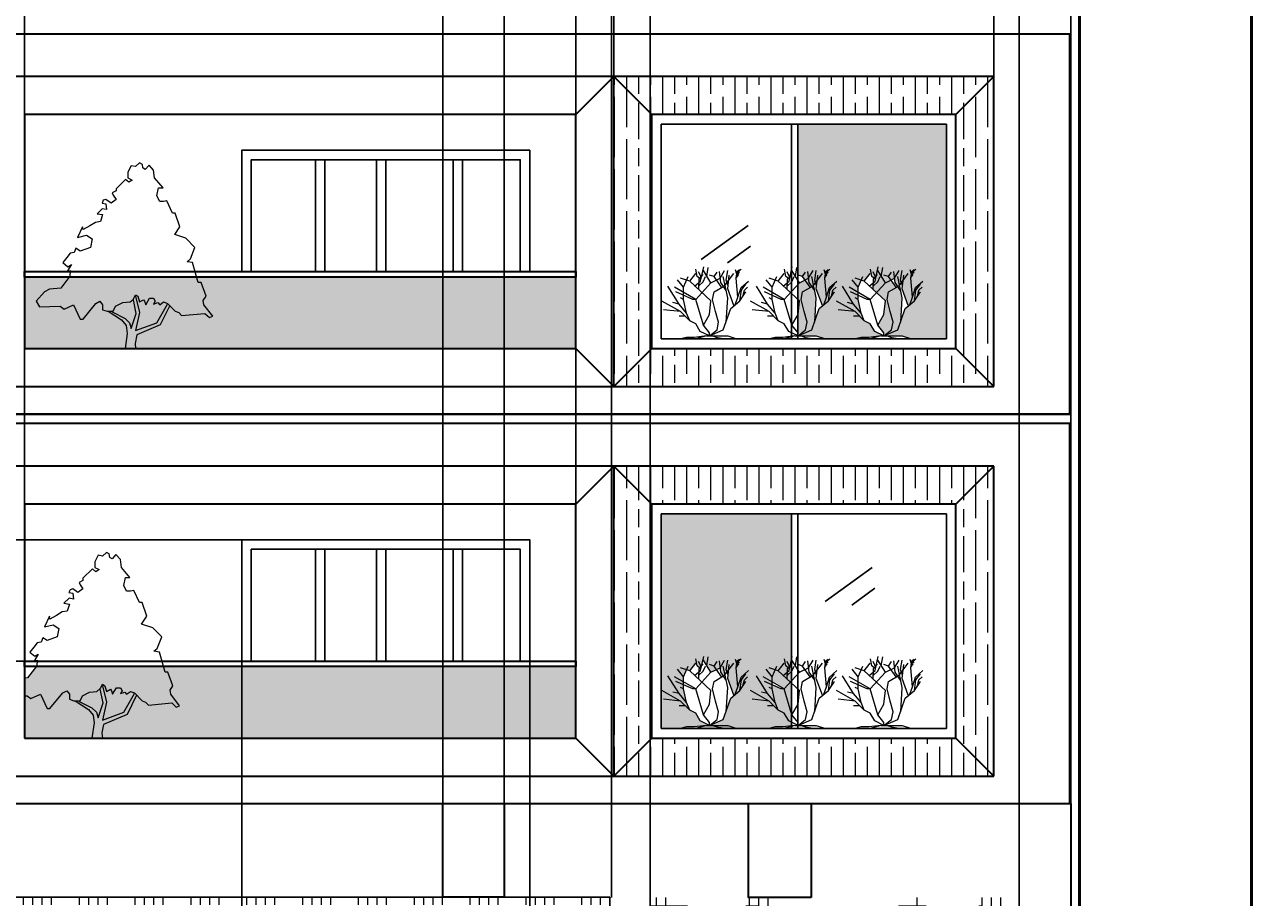
# Model space of a CAD drawing. Units: inches. Extents: x -97 to 1206, y -378 to 680.
# Tile 3 of 6: x 194 to 581, y -25 to 251. Entities that reach past the tile are written whole.
import ezdxf

# ---------------------------------------------------------------- set-up
doc = ezdxf.new("R2010")
doc.units = ezdxf.units.IN
doc.header["$MEASUREMENT"] = 0
for name, color, linetype, lineweight in [('A-ANNO-DIMS', 2, 'Continuous', 18), ('A-DOOR', 3, 'Continuous', 25), ('A-ELEV', 7, 'Continuous', 35), ('A-ELEV-PATT', 252, 'Continuous', 13), ('A-GLAZ', 4, 'Continuous', 25), ('A-WALL', 7, 'Continuous', 50), ('L-PLNT', 82, 'Continuous', 13)]:
    doc.layers.add(name, color=color, linetype=linetype, lineweight=lineweight)
doc.styles.get("Standard").update_dxf_attribs({"font": 'arial.ttf'})
doc.dimstyles.get("Standard").update_dxf_attribs({"dimtxt": 0.18, "dimasz": 0.18, "dimexe": 0.18, "dimexo": 0.0625, "dimgap": 0.09, "dimtad": 0, "dimtih": 1, "dimtoh": 1, "dimdec": 4, "dimzin": 0, "dimdsep": 46, "dimtxsty": 'Standard', "dimcen": 0.09, "dimadec": 0, "dimazin": 0, "dimtfac": 1, "dimtdec": 4, "dimtofl": 0, "dimtmove": 0, "dimatfit": 3, "dimfxl": 1, "dimtolj": 1, "dimtzin": 0, "dimarcsym": 0})
pattern_1 = [(45, (-208.809, -191.922), (8.48528, 0), [5, -7]), (45, (-206.6876, -191.922), (8.48528, 0), [2, -10]), (45, (-208.809, -189.8007), (8.48528, 0), [2, -10])]

# ---------------------------------------------------------------- blocks, each defined once
blk = doc.blocks.new('*U2')
for p, q in [((-16.8, 16.32), (-15.36, 19.68)), ((-14.88, 18.24), (-12.96, 20.64)), ((-12.471, 19.775), (-12.898, 22.044)), ((-11.677, 19.071), (-12.471, 19.775)), ((-11.28, 19.619), (-12.104, 21.184)), ((-11.921, 18.836), (-10.64, 20.401)), ((-11.433, 18.289), (-10.457, 22.749)), ((-10.579, 18.054), (-9.846, 19.697)), ((-8.16, 17.76), (-10.56, 21.6)), ((-9.48, 19.775), (-8.992, 22.592)), ((-7.2, 19.68), (-8.64, 20.16)), ((-7.2, 19.68), (-6.24, 21.12)), ((-4.8, 16.32), (-7.2, 19.68)), ((-5.086, 17.741), (-5.513, 21.34)), ((-5.28, 19.2), (-3.84, 21.6)), ((-2.88, 12.96), (-4.32, 19.68)), ((-3.84, 16.8), (-0.96, 20.64)), ((-3.377, 18.602), (-2.888, 21.575)), ((-2.88, 15.84), (-2.4, 20.16)), ((-0.508, 21.888), (-0.081, 20.558)), ((-0.203, 19.149), (0.102, 21.34)), ((-0.142, 19.384), (0.59, 20.401)), ((-0.02, 20.01), (0.896, 21.105)), ((0.041, 20.714), (1.384, 22.044)), ((0.102, 21.34), (0.835, 21.888)), ((-18.24, 11.04), (-21.755, 16.655)), ((-12.96, 12.48), (-19.68, 16.32)), ((-16.8, 16.32), (-18.72, 18.72)), ((-14.88, 18.24), (-17.76, 19.2)), ((-16.8, 12.48), (-16.8, 16.32)), ((-8.16, 12), (-14.88, 18.24)), ((-13.325, 16.724), (-11.433, 18.289)), ((-12.96, 12.48), (-8.16, 17.76)), ((-12.043, 15.628), (-11.921, 18.836)), ((-11.982, 16.802), (-10.579, 18.054)), ((-8.16, 17.76), (-5.28, 19.2)), ((-7.2, 14.88), (-3.84, 16.8)), ((-3.377, 15.315), (-5.086, 17.819)), ((-2.766, 16.802), (-3.377, 18.602)), ((-0.96, 10.56), (-2.88, 15.84)), ((0.346, 13.203), (-0.203, 19.149)), ((0.346, 13.203), (1.323, 16.254)), ((1.323, 16.254), (3.642, 18.289)), ((1.44, 15.36), (2.88, 17.28)), ((2.4, 15.36), (3.36, 16.32)), ((-17.76, 8.64), (-23.663, 11.961)), ((-13.92, 12.48), (-19.2, 14.88)), ((-16.8, 12.48), (-17.76, 12.96)), ((-15.84, 8.16), (-16.8, 12.48)), ((-12.96, 12.48), (-13.92, 12.48)), ((-10.56, 4.32), (-12.96, 12.48)), ((-8.64, 7.68), (-8.16, 12)), ((-7.68, 12.48), (-7.2, 14.88)), ((-6.72, 8.64), (-7.68, 12.48)), ((-3.36, 5.28), (-2.88, 12.96)), ((-1.92, 9.6), (0.96, 12)), ((-0.48, 10.8), (0.346, 13.203)), ((0.96, 12), (1.44, 15.36)), ((0.96, 12), (2.88, 14.88)), ((1.92, 13.44), (2.4, 15.36)), ((-17.76, 8.64), (-23.128, 9.222)), ((-18.24, 11.04), (-20.16, 11.52)), ((-15.84, 8.16), (-18.24, 11.04)), ((-14.88, 5.76), (-17.76, 8.64)), ((-14.88, 5.76), (-15.84, 8.16)), ((-5.76, 5.28), (-6.72, 8.64)), ((-4.32, 2.88), (-1.92, 9.6)), ((-16.32, 7.2), (-18.24, 7.2)), ((-12.96, 4.8), (-14.88, 5.76)), ((-11.52, 2.4), (-12.96, 4.8)), ((-10.56, 4.32), (-8.64, 7.68)), ((-8.64, 1.92), (-10.56, 4.32)), ((-6.24, 2.88), (-5.76, 5.28)), ((-15.84, 0.48), (-17.76, 0)), ((-13.44, 0.48), (-15.84, 0.48)), ((-9.6, 0.96), (-13.44, 0.48)), ((-9.6, 0.96), (-12.96, 0)), ((-8.64, 0.96), (-11.52, 2.4)), ((-9.6, 0.96), (-7.68, 0.96)), ((-8.64, 0.96), (-4.32, 2.88)), ((-8.64, 0.96), (-6.24, 2.88)), ((-8.64, 0.96), (-8.64, 1.92)), ((-8.64, 0.96), (-2.88, 0.96)), ((-7.68, 0.96), (-6.24, 0.48)), ((-6.24, 0.48), (-3.36, 0)), ((-2.88, 0.96), (0, 0))]:
    blk.add_line(p, q)
blk = doc.blocks.new('*U3')
for points in [[(22.0124, 137.721), (18.5475, 141.5624), (15.5282, 138.2446), (13.8028, 139.3505), (13.3714, 142.1153), (11.2148, 143.2214), (8.1954, 140.4564), (4.7447, 141.0094), (2.1567, 136.0326), (2.1567, 131.6088), (5.6074, 129.9499), (3.0193, 128.2909), (0.4313, 130.5029), (-6.9015, 123.3141), (-6.9015, 121.6552), (-9.9208, 119.9963), (-9.0581, 118.3373), (-6.9015, 115.0195), (-10.7835, 112.2546), (-14.6656, 115.0195), (-16.8222, 114.4665), (-17.6849, 112.2546), (-14.6656, 111.7016), (-14.2342, 107.2778), (-17.6065, 107.8307), (-21.5669, 103.9599), (-17.2536, 103.4069), (-18.9789, 97.8771), (-22.8609, 97.3241), (-27.1743, 94.5593), (-32.3504, 91.7944), (-32.7817, 94.0063), (-36.6638, 85.7116), (-29.7624, 87.3705), (-25.449, 84.6056), (-26.743, 77.9699), (-34.507, 75.205), (-37.9578, 77.4169), (-39.2518, 74.099), (-42.2711, 73.5461), (-44.8592, 70.2282), (-47.8786, 66.3574), (-43.9965, 63.0395), (-41.4085, 64.6985), (-44.3346, 59.8898), (-42.2089, 60.1377), (-42.5159, 55.7849), (-49.6039, 46.4502), (-58.2307, 45.8972), (-62.1127, 43.6853), (-68.5828, 36.4966), (-65.9947, 32.0727), (-50.0352, 32.6257), (-47.0159, 30.4138), (-39.6831, 33.7317), (-34.507, 22.6721), (-32.3504, 22.6721), (-22.4296, 34.8376), (-19.4102, 36.4966), (-17.2536, 33.7317), (-17.2536, 29.8608), (-13.8028, 28.7549), (-9.0581, 28.7549), (-7.3328, 32.6257), (-1.7254, 35.3906), (3.8821, 35.9436), (6.4701, 38.1555), (6.9014, 38.7085), (8.1954, 41.4734), (9.9208, 40.3674), (11.2148, 35.9436), (14.2341, 37.6025), (15.0968, 36.4966), (15.9595, 33.7317), (18.9789, 38.7085), (21.9982, 38.7085), (23.2922, 36.4966), (21.9982, 34.2847), (25.4489, 35.3906), (26.743, 33.7317), (29.7623, 35.9436), (32.7817, 34.8376), (38.8204, 28.7549), (41.4084, 27.6489), (43.5651, 25.437), (61.6813, 27.0959), (65.132, 23.7781), (67.7201, 24.884), (60.8186, 33.7317), (60.3873, 37.0495), (62.544, 40.3674), (58.662, 50.874), (56.5053, 50.874), (52.1919, 66.3574), (47.8785, 66.9103), (50.4665, 69.1222), (53.9172, 77.9699), (47.0158, 85.1586), (38.3891, 87.9235), (42.2711, 94.0063)], [(42.2711, 94.0063), (38.8204, 104.5129), (36.6637, 104.5129), (32.3503, 113.9135), (29.7623, 113.3605), (26.743, 113.3605), (24.5862, 117.7844), (25.8802, 123.8671), (29.331, 123.8671), (22.8609, 131.6088), (21.9982, 137.6916)], [(8.1954, 40.3674), (11.2148, 27.6489), (8.1954, 13.8245), (24.5862, 19.9072), (32.7817, 34.2847)], [(-12.9401, 28.7549), (-2.588, 22.1191), (0.8626, 17.6953), (1.7253, 11.6125), (0, 0)], [(-9.9208, 28.2019), (0, 23.2251), (3.4507, 19.9072), (4.7447, 15.4834), (8.6267, 27.0959), (6.4701, 37.6025)], [(34.5071, 33.1787), (27.1743, 18.2483), (9.0581, 10.5066), (7.7641, 3.8708), (8.1954, 0)]]:
    blk.add_lwpolyline(points)
blk = doc.blocks.new('FACADE-SURROUND')
for p, q in [((432, 97.83), (0, 97.83)), ((0, 97.83), (0, 0)), ((12, 85.83), (0, 97.83)), ((300, 85.83), (312, 97.83)), ((312, 0), (312, 97.83)), ((312, 0), (312, 97.83)), ((312, 97.83), (324, 85.83)), ((432, 97.83), (420, 85.83)), ((432, 0), (432, 97.83)), ((12, 85.83), (12, 12)), ((108, 85.83), (12, 85.83)), ((300, 85.83), (126, 85.83)), ((126, 85.83), (126, 12)), ((300, 12), (300, 85.83)), ((324, 12), (324, 85.83)), ((420, 85.83), (324, 85.83)), ((420, 12), (420, 85.83)), ((12, 12), (0, 0)), ((12, 12), (108, 12)), ((126, 12), (300, 12)), ((300, 12), (312, 0)), ((312, 0), (324, 12)), ((324, 12), (420, 12)), ((432, 0), (420, 12)), ((0, 0), (432, 0))]:
    blk.add_line(p, q)
blk = doc.blocks.new('WIN-1500')
for p, q in [((90, 67.83), (0, 67.83)), ((0, 67.83), (0, 0)), ((90, 67.83), (90, 0)), ((0, 0), (90, 0))]:
    blk.add_line(p, q)
blk = doc.blocks.new('*D21')
at = {"layer": 'A-ANNO-DIMS', "color": 0, "lineweight": -2, "transparency": 16777216}
for p, q in [((379.25, -24.78), (379.25, 679.54)), ((379.43, 679.36), (451.27, 679.36)), ((524.01, 679.36), (452.18, 679.36)), ((524.19, -24.78), (524.19, 679.54))]:
    blk.add_line(p, q, dxfattribs=at)
at = {"layer": 'A-ANNO-DIMS', "color": 0, "transparency": 16777216}
for points in [[(379.43, 679.39), (379.43, 679.33), (379.25, 679.36)], [(524.01, 679.39), (524.01, 679.33), (524.19, 679.36)]]:
    blk.add_solid(points, dxfattribs=at)
at = {"layer": 'Defpoints', "color": 0, "transparency": 16777216}
for p in [(524.19, 679.36), (379.25, -24.84), (524.19, -24.84)]:
    blk.add_point(p, dxfattribs=at)
at = {"layer": 'A-ANNO-DIMS', "color": 0, "transparency": 16777216, "insert": (451.72, 679.36), "char_height": 0.18, "attachment_point": 5}
blk.add_mtext('\\A1;144.94', dxfattribs=at)
blk = doc.blocks.new('*D38')
at = {"layer": 'A-ANNO-DIMS', "color": 0, "lineweight": -2, "transparency": 16777216}
for p, q in [((391.36, -84.5), (391.36, 679.54)), ((391.54, 679.36), (449.18, 679.36)), ((507.74, 679.36), (450.1, 679.36)), ((507.92, -84.5), (507.92, 679.54))]:
    blk.add_line(p, q, dxfattribs=at)
at = {"layer": 'A-ANNO-DIMS', "color": 0, "transparency": 16777216}
for points in [[(391.54, 679.39), (391.54, 679.33), (391.36, 679.36)], [(507.74, 679.39), (507.74, 679.33), (507.92, 679.36)]]:
    blk.add_solid(points, dxfattribs=at)
at = {"layer": 'Defpoints', "color": 0, "transparency": 16777216}
for p in [(507.92, 679.36), (391.36, -84.57), (507.92, -84.57)]:
    blk.add_point(p, dxfattribs=at)
at = {"layer": 'A-ANNO-DIMS', "color": 0, "transparency": 16777216, "insert": (449.64, 679.36), "char_height": 0.18, "attachment_point": 5}
blk.add_mtext('\\A1;116.56', dxfattribs=at)
blk = doc.blocks.new('*D40')
at = {"layer": 'A-ANNO-DIMS', "color": 0, "lineweight": -2, "transparency": 16777216}
for p, q in [((193.93, 99.46), (193.93, 679.54)), ((194.11, 679.36), (280.65, 679.36)), ((367.75, 679.36), (281.21, 679.36)), ((367.93, 99.46), (367.93, 679.54))]:
    blk.add_line(p, q, dxfattribs=at)
at = {"layer": 'A-ANNO-DIMS', "color": 0, "transparency": 16777216}
for points in [[(194.11, 679.39), (194.11, 679.33), (193.93, 679.36)], [(367.75, 679.39), (367.75, 679.33), (367.93, 679.36)]]:
    blk.add_solid(points, dxfattribs=at)
at = {"layer": 'Defpoints', "color": 0, "transparency": 16777216}
for p in [(367.93, 679.36), (193.93, 99.4), (367.93, 99.4)]:
    blk.add_point(p, dxfattribs=at)
at = {"layer": 'A-ANNO-DIMS', "color": 0, "transparency": 16777216, "insert": (280.93, 679.36), "char_height": 0.18, "attachment_point": 5}
blk.add_mtext('\\A1;174', dxfattribs=at)
blk = doc.blocks.new('*D43')
at = {"layer": 'A-ANNO-DIMS', "color": 0, "lineweight": -2, "transparency": 16777216}
for p, q in [((262.49, 49.82), (262.49, -377.59)), ((353.38, 49.82), (353.38, -377.59)), ((262.67, -377.41), (307.54, -377.41)), ((353.2, -377.41), (308.33, -377.41))]:
    blk.add_line(p, q, dxfattribs=at)
at = {"layer": 'A-ANNO-DIMS', "color": 0, "transparency": 16777216}
for points in [[(262.67, -377.38), (262.67, -377.44), (262.49, -377.41)], [(353.2, -377.38), (353.2, -377.44), (353.38, -377.41)]]:
    blk.add_solid(points, dxfattribs=at)
at = {"layer": 'Defpoints', "color": 0, "transparency": 16777216}
for p in [(262.49, 49.88), (353.38, 49.88), (353.38, -377.41)]:
    blk.add_point(p, dxfattribs=at)
at = {"layer": 'A-ANNO-DIMS', "color": 0, "transparency": 16777216, "insert": (307.94, -377.41), "char_height": 0.18, "attachment_point": 5}
blk.add_mtext('\\A1;90.88', dxfattribs=at)
blk = doc.blocks.new('*D44')
at = {"layer": 'A-ANNO-DIMS', "color": 0, "lineweight": -2, "transparency": 16777216}
for p, q in [((262.43, 88.15), (-96.59, 88.15)), ((-96.41, 87.97), (-96.41, 69.2)), ((-96.41, 50.06), (-96.41, 68.83)), ((262.43, 49.88), (-96.59, 49.88))]:
    blk.add_line(p, q, dxfattribs=at)
at = {"layer": 'A-ANNO-DIMS', "color": 0, "transparency": 16777216}
for points in [[(-96.44, 87.97), (-96.38, 87.97), (-96.41, 88.15)], [(-96.44, 50.06), (-96.38, 50.06), (-96.41, 49.88)]]:
    blk.add_solid(points, dxfattribs=at)
at = {"layer": 'Defpoints', "color": 0, "transparency": 16777216}
for p in [(-96.41, 88.15), (262.49, 88.15), (262.49, 49.88)]:
    blk.add_point(p, dxfattribs=at)
at = {"layer": 'A-ANNO-DIMS', "color": 0, "transparency": 16777216, "insert": (-96.41, 69.01), "char_height": 0.18, "attachment_point": 5}
blk.add_mtext('\\A1;38.266', dxfattribs=at)
blk = doc.blocks.new('*D47')
at = {"layer": 'A-ANNO-DIMS', "color": 0, "lineweight": -2, "transparency": 16777216}
for p, q in [((184.83, -24.66), (184.83, 679.54)), ((185.01, 679.36), (255.01, 679.36)), ((325.75, 679.36), (255.75, 679.36)), ((325.93, -24.66), (325.93, 679.54))]:
    blk.add_line(p, q, dxfattribs=at)
at = {"layer": 'A-ANNO-DIMS', "color": 0, "transparency": 16777216}
for points in [[(185.01, 679.39), (185.01, 679.33), (184.83, 679.36)], [(325.75, 679.39), (325.75, 679.33), (325.93, 679.36)]]:
    blk.add_solid(points, dxfattribs=at)
at = {"layer": 'Defpoints', "color": 0, "transparency": 16777216}
for p in [(325.93, 679.36), (184.83, -24.73), (325.93, -24.73)]:
    blk.add_point(p, dxfattribs=at)
at = {"layer": 'A-ANNO-DIMS', "color": 0, "transparency": 16777216, "insert": (255.38, 679.36), "char_height": 0.18, "attachment_point": 5}
blk.add_mtext('\\A1;141.1', dxfattribs=at)
blk = doc.blocks.new('*D48')
at = {"layer": 'A-ANNO-DIMS', "color": 0, "lineweight": -2, "transparency": 16777216}
for p, q in [((325.93, -24.66), (325.93, 679.54)), ((326.11, 679.36), (335.23, 679.36)), ((345.13, 679.36), (336, 679.36)), ((345.31, -24.66), (345.31, 679.54))]:
    blk.add_line(p, q, dxfattribs=at)
at = {"layer": 'A-ANNO-DIMS', "color": 0, "transparency": 16777216}
for points in [[(326.11, 679.39), (326.11, 679.33), (325.93, 679.36)], [(345.13, 679.39), (345.13, 679.33), (345.31, 679.36)]]:
    blk.add_solid(points, dxfattribs=at)
at = {"layer": 'Defpoints', "color": 0, "transparency": 16777216}
for p in [(345.31, 679.36), (325.93, -24.73), (345.31, -24.73)]:
    blk.add_point(p, dxfattribs=at)
at = {"layer": 'A-ANNO-DIMS', "color": 0, "transparency": 16777216, "insert": (335.62, 679.36), "char_height": 0.18, "attachment_point": 5}
blk.add_mtext('\\A1;19.38', dxfattribs=at)
blk = doc.blocks.new('*D58')
at = {"layer": 'A-ANNO-DIMS', "color": 0, "lineweight": -2, "transparency": 16777216}
for p, q in [((379.93, 234.46), (379.93, 679.54)), ((380.11, 679.36), (439.47, 679.36)), ((499.75, 679.36), (440.38, 679.36)), ((499.93, 234.46), (499.93, 679.54))]:
    blk.add_line(p, q, dxfattribs=at)
at = {"layer": 'A-ANNO-DIMS', "color": 0, "transparency": 16777216}
for points in [[(380.11, 679.39), (380.11, 679.33), (379.93, 679.36)], [(499.75, 679.39), (499.75, 679.33), (499.93, 679.36)]]:
    blk.add_solid(points, dxfattribs=at)
at = {"layer": 'Defpoints', "color": 0, "transparency": 16777216}
for p in [(499.93, 679.36), (379.93, 234.4), (499.93, 234.4)]:
    blk.add_point(p, dxfattribs=at)
at = {"layer": 'A-ANNO-DIMS', "color": 0, "transparency": 16777216, "insert": (439.93, 679.36), "char_height": 0.18, "attachment_point": 5}
blk.add_mtext('\\A1;120.00', dxfattribs=at)

msp = doc.modelspace()

# ---------------------------------------------------------------- hatches: boundary and pattern name
at = {"layer": 'A-ELEV-PATT'}
h = msp.add_hatch(dxfattribs=at)
h.set_pattern_fill('GOST_GLASS', color=256)
h.set_pattern_definition(pattern_1)
h.paths.add_polyline_path([(441.8335, 588.3966), (394.9261, 588.3966), (394.9261, 520.5671), (441.8335, 520.5671)])
h.paths.add_polyline_path([(484.9261, 465.3966), (443.8021, 465.3966), (443.8021, 397.5671), (484.9261, 397.5671)])
h.paths.add_polyline_path([(441.8335, 342.3966), (394.9261, 342.3966), (394.9261, 274.5671), (441.8335, 274.5671)])
h.paths.add_polyline_path([(484.9261, 219.3966), (438.0187, 219.3966), (438.0187, 171.7458), (439.5149, 171.2471), (440.2728, 170.186), (438.5549, 169.3271), (438.0187, 168.7372), (438.0187, 164.065), (438.5549, 163.5671), (438.0187, 158.741), (438.0187, 153.5574), (438.6415, 152.7789), (438.0749, 152.5271), (443.8349, 152.5271), (446.7149, 151.5671), (456.0952, 151.5671), (458.0152, 152.0471), (460.4152, 152.0471), (465.0232, 152.6231), (462.3352, 153.9671), (460.8952, 156.3671), (458.9752, 157.3271), (458.0152, 159.7271), (457.0552, 164.0471), (457.0552, 167.8871), (458.0152, 170.1271), (458.9752, 169.8071), (461.1593, 172.5372), (461.3842, 171.3421), (462.1483, 170.6646), (462.7637, 171.4165), (462.4222, 169.8561), (461.8969, 169.4216), (461.8114, 167.1735), (465.6952, 163.5671), (465.2152, 159.2471), (463.2952, 155.8871), (465.7818, 152.7789), (465.2152, 152.5271), (470.9752, 152.5271), (473.8552, 151.5671), (484.9261, 151.5671)])
h.paths.add_polyline_path([(473.7595, 171.4865), (473.9183, 171.6764), (473.8259, 171.964)], flags=16)
h.paths.add_polyline_path([(468.5752, 170.7671), (468.5927, 170.7962), (468.758, 169.4025), (469.6192, 168.1408), (470.0152, 168.3671), (471.2674, 170.0367), (470.9752, 167.4071), (472.9399, 162.0043), (471.9352, 161.1671), (470.517, 157.1962), (470.9752, 164.5271), (470.4671, 166.8984), (469.6192, 168.1408), (469.09, 167.8384), (467.4131, 170.186)], flags=16)
h.paths.add_polyline_path([(446.6192, 171.4865), (446.778, 171.6764), (446.6857, 171.964)], flags=16)
h.paths.add_polyline_path([(444.7949, 161.1671), (443.3768, 157.1962), (443.8349, 164.5271), (443.3268, 166.8984), (442.4789, 168.1408), (442.8749, 168.3671), (444.1271, 170.0367), (443.8349, 167.4071), (445.7996, 162.0043)], flags=16)
h.paths.add_polyline_path([(436.0501, 96.3966), (394.9261, 96.3966), (394.9261, 28.5671), (436.0501, 28.5671)])
h.paths.add_polyline_path([(418.6647, 48.4865), (418.8235, 48.6764), (418.7312, 48.964)], flags=16)
h.paths.add_polyline_path([(408.0905, 50.343), (410.6005, 46.3271), (413.4805, 47.7671), (413.4979, 47.7962), (413.6633, 46.4025), (414.5244, 45.1408), (414.9205, 45.3671), (416.1726, 47.0367), (415.8805, 44.4071), (417.8451, 39.0043), (416.8405, 38.1671), (414.4405, 31.4471), (410.1205, 29.5271), (407.2405, 30.9671), (405.8005, 33.3671), (403.8805, 34.3271), (402.9205, 36.7271), (401.9605, 41.0471), (401.9605, 44.8871), (402.9205, 47.1271), (403.8805, 46.8071), (406.0646, 49.5372), (406.2895, 48.3421), (407.0535, 47.6646), (407.6689, 48.4165)], flags=16)
h.paths.add_polyline_path([(406.7167, 44.1735), (410.6005, 40.5671), (410.1205, 36.2471), (408.2005, 32.8871), (405.8005, 41.0471), (407.761, 43.2037), (405.4765, 45.3251), (406.8021, 46.4216)], flags=0)
h.paths.add_polyline_path([(429.9149, 43.2414), (433.7549, 41.0471), (432.7949, 41.0471), (429.9149, 42.3562)], flags=16)
h = msp.add_hatch(dxfattribs=at)
h.set_pattern_fill('GOST_GLASS', color=256)
h.set_pattern_definition(pattern_1)
h.paths.add_polyline_path([(225.9926, 155.8067), (224.5809, 157.6166), (220.3456, 160.3315), (219.9926, 160.3315), (218.5808, 160.7839), (218.5808, 162.3676), (217.6985, 163.4988), (216.4631, 162.8201), (212.4043, 157.8428), (211.522, 157.8428), (209.4043, 162.3676), (206.4043, 161.0102), (205.169, 161.9151), (198.6395, 161.6889), (197.5807, 163.4988), (200.2278, 166.4399), (201.816, 167.3448), (205.3454, 167.5711), (208.0494, 171.1321), (193.9261, 171.1321), (193.9261, 148.5671), (225.6397, 148.5671), (226.3455, 153.3181)])
h.paths.add_polyline_path([(228.9926, 165.5349), (229.6985, 165.0825), (230.2279, 163.2726), (231.4632, 163.9513), (231.8162, 163.4988), (232.1691, 162.3676), (233.4044, 164.4038), (234.6397, 164.4038), (235.1691, 163.4988), (234.6397, 162.5939), (236.0515, 163.0463), (236.5809, 162.3676), (237.8162, 163.2726), (239.0515, 162.8201), (241.5221, 160.3315), (242.5809, 159.879), (243.4633, 158.974), (250.8751, 159.6527), (252.2869, 158.2953), (253.3457, 158.7478), (250.5222, 162.3676), (250.3457, 163.725), (251.2281, 165.0825), (249.6398, 169.381), (248.7575, 169.381), (248.2696, 171.1321), (208.0494, 171.1321), (205.3454, 167.5711), (201.816, 167.3448), (200.2278, 166.4399), (197.5807, 163.4988), (198.6395, 161.6889), (205.169, 161.9151), (206.4043, 161.0102), (209.4043, 162.3676), (211.522, 157.8428), (212.4043, 157.8428), (216.4631, 162.8201), (217.6985, 163.4988), (218.5808, 162.3676), (218.5808, 160.7839), (219.9926, 160.3315), (221.9338, 160.3315), (222.6396, 161.9151), (224.9338, 163.0463), (227.228, 163.2726), (228.2868, 164.1775), (228.4632, 164.4038)])
h.paths.add_polyline_path([(236.7574, 156.033), (239.7468, 162.1197), (239.0515, 162.8201), (237.8162, 163.2726), (236.5809, 162.3676), (236.0515, 163.0463), (234.6397, 162.5939), (235.1691, 163.4988), (234.6397, 164.4038), (233.4044, 164.4038), (232.1691, 162.3676), (231.8162, 163.4988), (231.4632, 163.9513), (230.2279, 163.2726), (229.6985, 165.0825), (228.9926, 165.5349), (228.4632, 164.4038), (228.2868, 164.1775), (227.228, 163.2726), (224.9338, 163.0463), (222.6396, 161.9151), (221.9338, 160.3315), (220.3456, 160.3315), (224.5809, 157.6166), (225.9926, 155.8067), (226.3455, 153.3181), (225.6397, 148.5671), (228.9926, 148.5671), (228.8162, 150.1507), (229.3456, 152.8656)])
h.paths.add_polyline_path([(367.9261, 171.1321), (248.2696, 171.1321), (248.7575, 169.381), (249.6398, 169.381), (251.2281, 165.0825), (250.3457, 163.725), (250.5222, 162.3676), (253.3457, 158.7478), (252.2869, 158.2953), (250.8751, 159.6527), (243.4633, 158.974), (242.5809, 159.879), (241.5221, 160.3315), (239.7468, 162.1197), (236.7574, 156.033), (229.3456, 152.8656), (228.8162, 150.1507), (228.9926, 148.5671), (367.9261, 148.5671)])
h.paths.add_polyline_path([(367.9261, 48.1321), (237.8147, 48.1321), (238.3026, 46.381), (239.1849, 46.381), (240.7732, 42.0825), (239.8908, 40.725), (240.0673, 39.3676), (242.8908, 35.7478), (241.832, 35.2953), (240.4202, 36.6527), (233.0084, 35.974), (232.126, 36.879), (231.0672, 37.3315), (229.2919, 39.1197), (226.3025, 33.033), (218.8907, 29.8656), (218.3613, 27.1507), (218.5377, 25.5671), (367.9261, 25.5671)])
h.paths.add_polyline_path([(226.3025, 33.033), (229.2919, 39.1197), (228.5966, 39.8201), (227.3613, 40.2726), (226.126, 39.3676), (225.5966, 40.0463), (224.1848, 39.5939), (224.7142, 40.4988), (224.1848, 41.4038), (222.9495, 41.4038), (221.7142, 39.3676), (221.3613, 40.4988), (221.0083, 40.9513), (219.7731, 40.2726), (219.2436, 42.0825), (218.5377, 42.5349), (218.0083, 41.4038), (217.8319, 41.1775), (216.7731, 40.2726), (214.4789, 40.0463), (212.1847, 38.9151), (211.4789, 37.3315), (209.8907, 37.3315), (214.126, 34.6166), (215.5377, 32.8067), (215.8907, 30.3181), (215.1848, 25.5671), (218.5377, 25.5671), (218.3613, 27.1507), (218.8907, 29.8656)])
h.paths.add_polyline_path([(239.1849, 46.381), (238.3026, 46.381), (237.8147, 48.1321), (197.5945, 48.1321), (194.8905, 44.5711), (193.9261, 44.5093), (193.9261, 38.8878), (194.7141, 38.9151), (195.9494, 38.0102), (198.9494, 39.3676), (201.0671, 34.8428), (201.9494, 34.8428), (206.0083, 39.8201), (207.2436, 40.4988), (208.1259, 39.3676), (208.1259, 37.7839), (209.5377, 37.3315), (211.4789, 37.3315), (212.1847, 38.9151), (214.4789, 40.0463), (216.7731, 40.2726), (217.8319, 41.1775), (218.0083, 41.4038), (218.5377, 42.5349), (219.2436, 42.0825), (219.7731, 40.2726), (221.0083, 40.9513), (221.3613, 40.4988), (221.7142, 39.3676), (222.9495, 41.4038), (224.1848, 41.4038), (224.7142, 40.4988), (224.1848, 39.5939), (225.5966, 40.0463), (226.126, 39.3676), (227.3613, 40.2726), (228.5966, 39.8201), (231.0672, 37.3315), (232.126, 36.879), (233.0084, 35.974), (240.4202, 36.6527), (241.832, 35.2953), (242.8908, 35.7478), (240.0673, 39.3676), (239.8908, 40.725), (240.7732, 42.0825)])
h.paths.add_polyline_path([(215.5377, 32.8067), (214.126, 34.6166), (209.8907, 37.3315), (209.5377, 37.3315), (208.1259, 37.7839), (208.1259, 39.3676), (207.2436, 40.4988), (206.0083, 39.8201), (201.9494, 34.8428), (201.0671, 34.8428), (198.9494, 39.3676), (195.9494, 38.0102), (194.7141, 38.9151), (193.9261, 38.8878), (193.9261, 25.5671), (215.1848, 25.5671), (215.8907, 30.3181)])
h.paths.add_polyline_path([(336.7518, 280.6166), (332.5165, 283.3315), (332.1636, 283.3315), (330.7518, 283.7839), (330.7518, 285.3676), (329.8694, 286.4988), (328.6341, 285.8201), (324.5753, 280.8428), (323.6929, 280.8428), (321.5753, 285.3676), (318.5752, 284.0102), (317.3399, 284.9151), (310.8105, 284.6889), (309.7516, 286.4988), (312.3987, 289.4399), (313.987, 290.3448), (317.5164, 290.5711), (320.2203, 294.1321), (199.9261, 294.1321), (199.9261, 271.5671), (337.8106, 271.5671), (338.5165, 276.3181), (338.1636, 278.8067)])
h.paths.add_polyline_path([(321.5753, 408.3676), (318.5752, 407.0102), (317.3399, 407.9151), (310.8105, 407.6889), (309.7516, 409.4988), (312.3987, 412.4399), (313.987, 413.3448), (317.5164, 413.5711), (320.2203, 417.1321), (199.9261, 417.1321), (199.9261, 394.5671), (337.8106, 394.5671), (338.5165, 399.3181), (338.1636, 401.8067), (336.7518, 403.6166), (332.5165, 406.3315), (332.1636, 406.3315), (330.7518, 406.7839), (330.7518, 408.3676), (329.8694, 409.4988), (328.6341, 408.8201), (324.5753, 403.8428), (323.6929, 403.8428)])
h.paths.add_polyline_path([(373.9261, 540.1321), (79.9261, 540.1321), (79.9261, 517.5671), (373.9261, 517.5671)])
h.paths.add_polyline_path([(373.9261, 417.1321), (360.4406, 417.1321), (360.9284, 415.381), (361.8108, 415.381), (363.399, 411.0825), (362.5167, 409.725), (362.6931, 408.3676), (365.5167, 404.7478), (364.4578, 404.2953), (363.0461, 405.6527), (355.6343, 404.974), (354.7519, 405.879), (353.6931, 406.3315), (351.9178, 408.1197), (348.9284, 402.033), (341.5166, 398.8656), (340.9871, 396.1507), (341.1636, 394.5671), (373.9261, 394.5671)])
h.paths.add_polyline_path([(361.8108, 415.381), (360.9284, 415.381), (360.4406, 417.1321), (320.2203, 417.1321), (317.5164, 413.5711), (313.987, 413.3448), (312.3987, 412.4399), (309.7516, 409.4988), (310.8105, 407.6889), (317.3399, 407.9151), (318.5752, 407.0102), (321.5753, 408.3676), (323.6929, 403.8428), (324.5753, 403.8428), (328.6341, 408.8201), (329.8694, 409.4988), (330.7518, 408.3676), (330.7518, 406.7839), (332.1636, 406.3315), (334.1047, 406.3315), (334.8106, 407.9151), (337.1047, 409.0463), (339.3989, 409.2726), (340.4577, 410.1775), (340.6342, 410.4038), (341.1636, 411.5349), (341.8695, 411.0825), (342.3989, 409.2726), (343.6342, 409.9513), (343.9871, 409.4988), (344.3401, 408.3676), (345.5754, 410.4038), (346.8107, 410.4038), (347.3401, 409.4988), (346.8107, 408.5939), (348.2225, 409.0463), (348.7519, 408.3676), (349.9872, 409.2726), (351.2225, 408.8201), (353.6931, 406.3315), (354.7519, 405.879), (355.6343, 404.974), (363.0461, 405.6527), (364.4578, 404.2953), (365.5167, 404.7478), (362.6931, 408.3676), (362.5167, 409.725), (363.399, 411.0825)])
h.paths.add_polyline_path([(351.9178, 408.1197), (351.2225, 408.8201), (349.9872, 409.2726), (348.7519, 408.3676), (348.2225, 409.0463), (346.8107, 408.5939), (347.3401, 409.4988), (346.8107, 410.4038), (345.5754, 410.4038), (344.3401, 408.3676), (343.9871, 409.4988), (343.6342, 409.9513), (342.3989, 409.2726), (341.8695, 411.0825), (341.1636, 411.5349), (340.6342, 410.4038), (340.4577, 410.1775), (339.3989, 409.2726), (337.1047, 409.0463), (334.8106, 407.9151), (334.1047, 406.3315), (332.5165, 406.3315), (336.7518, 403.6166), (338.1636, 401.8067), (338.5165, 399.3181), (337.8106, 394.5671), (341.1636, 394.5671), (340.9871, 396.1507), (341.5166, 398.8656), (348.9284, 402.033)])
h.paths.add_polyline_path([(363.399, 288.0825), (361.8108, 292.381), (360.9284, 292.381), (360.4406, 294.1321), (320.2203, 294.1321), (317.5164, 290.5711), (313.987, 290.3448), (312.3987, 289.4399), (309.7516, 286.4988), (310.8105, 284.6889), (317.3399, 284.9151), (318.5752, 284.0102), (321.5753, 285.3676), (323.6929, 280.8428), (324.5753, 280.8428), (328.6341, 285.8201), (329.8694, 286.4988), (330.7518, 285.3676), (330.7518, 283.7839), (332.1636, 283.3315), (334.1047, 283.3315), (334.8106, 284.9151), (337.1047, 286.0463), (339.3989, 286.2726), (340.4577, 287.1775), (340.6342, 287.4038), (341.1636, 288.5349), (341.8695, 288.0825), (342.3989, 286.2726), (343.6342, 286.9513), (343.9871, 286.4988), (344.3401, 285.3676), (345.5754, 287.4038), (346.8107, 287.4038), (347.3401, 286.4988), (346.8107, 285.5939), (348.2225, 286.0463), (348.7519, 285.3676), (349.9872, 286.2726), (351.2225, 285.8201), (353.6931, 283.3315), (354.7519, 282.879), (355.6343, 281.974), (363.0461, 282.6527), (364.4578, 281.2953), (365.5167, 281.7478), (362.6931, 285.3676), (362.5167, 286.725)])
h.paths.add_polyline_path([(373.9261, 294.1321), (360.4406, 294.1321), (360.9284, 292.381), (361.8108, 292.381), (363.399, 288.0825), (362.5167, 286.725), (362.6931, 285.3676), (365.5167, 281.7478), (364.4578, 281.2953), (363.0461, 282.6527), (355.6343, 281.974), (354.7519, 282.879), (353.6931, 283.3315), (351.9178, 285.1197), (348.9284, 279.033), (341.5166, 275.8656), (340.9871, 273.1507), (341.1636, 271.5671), (373.9261, 271.5671)])
h.paths.add_polyline_path([(348.9284, 279.033), (351.9178, 285.1197), (351.2225, 285.8201), (349.9872, 286.2726), (348.7519, 285.3676), (348.2225, 286.0463), (346.8107, 285.5939), (347.3401, 286.4988), (346.8107, 287.4038), (345.5754, 287.4038), (344.3401, 285.3676), (343.9871, 286.4988), (343.6342, 286.9513), (342.3989, 286.2726), (341.8695, 288.0825), (341.1636, 288.5349), (340.6342, 287.4038), (340.4577, 287.1775), (339.3989, 286.2726), (337.1047, 286.0463), (334.8106, 284.9151), (334.1047, 283.3315), (332.5165, 283.3315), (336.7518, 280.6166), (338.1636, 278.8067), (338.5165, 276.3181), (337.8106, 271.5671), (341.1636, 271.5671), (340.9871, 273.1507), (341.5166, 275.8656)])
h = msp.add_hatch(dxfattribs=at)
h.set_pattern_fill('GOST_WOOD', color=256, scale=1.9)
h.set_pattern_definition([(90, (-208.809, -191.922), (11.4, -7e-16), [19, -3.8]), (90, (-205.009, -195.722), (11.4, -7e-16), [11.4, -2.85, 5.7, -2.85]), (90, (-201.209, -201.422), (11.4, -7e-16), [19, -3.8])])
h.paths.add_polyline_path([(499.9261, 111.3966), (379.9261, 111.3966), (391.9261, 99.3966), (487.9261, 99.3966)])
h.paths.add_polyline_path([(499.9261, 111.3966), (487.9261, 99.3966), (487.9261, 25.5671), (499.9261, 13.5671)])
h.paths.add_polyline_path([(487.9261, 25.5671), (391.9261, 25.5671), (379.9261, 13.5671), (499.9261, 13.5671)])
h.paths.add_polyline_path([(391.9261, 99.3966), (379.9261, 111.3966), (379.9261, 13.5671), (391.9261, 25.5671)])
h.paths.add_polyline_path([(391.9261, 222.3966), (379.9261, 234.3966), (379.9261, 136.5671), (391.9261, 148.5671)])
h.paths.add_polyline_path([(487.9261, 148.5671), (391.9261, 148.5671), (379.9261, 136.5671), (499.9261, 136.5671)])
h.paths.add_polyline_path([(499.9261, 234.3966), (487.9261, 222.3966), (487.9261, 148.5671), (499.9261, 136.5671)])
h.paths.add_polyline_path([(499.9261, 234.3966), (379.9261, 234.3966), (391.9261, 222.3966), (487.9261, 222.3966)])
h.paths.add_polyline_path([(187.9261, 357.3966), (67.9261, 357.3966), (79.9261, 345.3966), (175.9261, 345.3966)])
h.paths.add_polyline_path([(79.9261, 345.3966), (67.9261, 357.3966), (67.9261, 259.5671), (79.9261, 271.5671)])
h.paths.add_polyline_path([(175.9261, 271.5671), (79.9261, 271.5671), (67.9261, 259.5671), (187.9261, 259.5671)])
h.paths.add_polyline_path([(187.9261, 357.3966), (175.9261, 345.3966), (175.9261, 271.5671), (187.9261, 259.5671)])
h.paths.add_polyline_path([(79.9261, 468.3966), (67.9261, 480.3966), (67.9261, 382.5671), (79.9261, 394.5671)])
h.paths.add_polyline_path([(175.9261, 394.5671), (79.9261, 394.5671), (67.9261, 382.5671), (187.9261, 382.5671)])
h.paths.add_polyline_path([(187.9261, 480.3966), (67.9261, 480.3966), (79.9261, 468.3966), (175.9261, 468.3966)])
h.paths.add_polyline_path([(187.9261, 480.3966), (175.9261, 468.3966), (175.9261, 394.5671), (187.9261, 382.5671)])
h = msp.add_hatch(dxfattribs=at)
h.set_pattern_fill('HOUND', color=256, scale=47)
h.set_pattern_definition([(0, (-208.809, -191.922), (11.75, 2.9375), [47, -23.5]), (90, (-208.809, -191.922), (-2.9375, -11.75), [47, -23.5])])
h.paths.add_polyline_path([(81.8295, -48.3264), (-19.6789, -48.3264), (-19.6789, -97.3647), (81.8295, -97.3647)])
h.paths.add_polyline_path([(-8.2183, -60.8667), (63.8199, -60.8667), (63.8199, -84.3116), (-8.2183, -84.3116)], flags=16)
h.paths.add_polyline_path([(403.1688, -24.8426), (391.3618, -24.8426), (391.3618, -84.5669), (507.9182, -84.5669), (507.9182, -24.8426), (495.2029, -24.8426), (495.2029, -75.7956), (403.1688, -75.7956)])
h.paths.add_polyline_path([(430.113, -24.8426), (421.6362, -24.8426), (421.6362, -57.6481), (478.552, -57.6481), (478.552, -24.8426), (469.7725, -24.8426), (469.7725, -49.4817), (430.113, -49.4817)], flags=17)
h.paths.add_polyline_path([(378.6527, -24.7259), (98.5594, -24.7259), (98.5594, -27.0887), (378.6527, -27.0887)])
h.paths.add_polyline_path([(177.3114, -53.6191), (173.9058, -53.6191), (173.9058, -63.7423), (177.3114, -63.7423)])
h.paths.add_polyline_path([(177.3114, -63.7423), (173.9058, -63.7423), (173.9058, -69.9353), (177.3114, -69.9353)])
h.paths.add_polyline_path([(290.4371, -69.9353), (286.815, -69.9353), (286.815, -74.3824), (290.4371, -74.3824)])
h.paths.add_polyline_path([(290.4371, -63.7423), (286.815, -63.7423), (286.815, -69.9353), (290.4371, -69.9353)])
h.paths.add_polyline_path([(290.4371, -53.6191), (286.815, -53.6191), (286.815, -63.7423), (290.4371, -63.7423)])
h.paths.add_polyline_path([(290.4371, -50.7545), (286.815, -50.7545), (286.815, -53.6191), (290.4371, -53.6191)])

# ---------------------------------------------------------------- linework, layer by layer
at = {"layer": 'A-DOOR'}
msp.add_lwpolyline([(98.5594, -24.7259), (378.6527, -24.7259), (378.6527, -115.1448), (98.5594, -115.1448)], close=True, dxfattribs=at)
at = {"layer": 'A-ELEV'}
for p, q in [((523.9261, 247.8552), (46.9261, 247.8552)), ((523.9261, 127.8552), (523.9261, 247.8552)), ((262.4936, 172.8815), (353.3784, 172.8815)), ((523.9261, 127.8552), (46.9261, 127.8552)), ((46.9261, 127.8552), (523.9261, 127.8552)), ((523.9261, 124.8552), (46.9261, 124.8552)), ((523.9261, 4.8552), (523.9261, 124.8552)), ((262.4936, 49.8815), (353.3784, 49.8815)), ((46.9261, 4.8552), (523.9261, 4.8552))]:
    msp.add_line(p, q, dxfattribs=at)
for points in [[(523.9261, 127.8552), (523.9261, 247.8552)], [(523.9261, 4.8552), (523.9261, 124.8552)], [(46.9261, 4.8552), (524.19, 4.8552), (524.19, -115.1448), (43.9261, -115.1448)]]:
    msp.add_lwpolyline(points, dxfattribs=at)
for points in [[(193.9261, 172.8815), (367.9261, 172.8815), (367.9261, 171.1321), (193.9261, 171.1321)], [(193.9261, 49.8815), (367.9261, 49.8815), (367.9261, 48.1321), (193.9261, 48.1321)], [(345.3073, -24.7259), (325.9258, -24.7259), (325.9258, 4.8552), (345.3073, 4.8552)], [(442.2146, -24.8426), (422.4455, -24.8426), (422.4455, 4.8552), (442.2146, 4.8552)]]:
    msp.add_lwpolyline(points, close=True, dxfattribs=at)
at = {"layer": 'A-GLAZ'}
for p, q in [((407.4572, 176.6989), (422.3146, 187.3556)), ((415.8383, 175.5571), (423.0765, 180.8855)), ((446.6712, 68.6989), (461.5285, 79.3556)), ((455.0522, 67.5571), (462.2904, 72.8855))]:
    msp.add_line(p, q, dxfattribs=at)
for points in [[(436.0501, 219.3966), (438.0187, 219.3966), (438.0187, 151.5671), (436.0501, 151.5671)], [(285.8181, 208.1471), (288.7671, 208.1471), (288.7671, 172.8815), (285.8181, 172.8815)], [(304.987, 208.1471), (307.936, 208.1471), (307.936, 172.8815), (304.987, 172.8815)], [(329.2497, 208.1471), (332.1988, 208.1471), (332.1988, 172.8815), (329.2497, 172.8815)], [(436.0501, 96.3966), (438.0187, 96.3966), (438.0187, 28.5671), (436.0501, 28.5671)], [(285.8181, 85.1471), (288.7671, 85.1471), (288.7671, 49.8815), (285.8181, 49.8815)], [(304.987, 85.1471), (307.936, 85.1471), (307.936, 49.8815), (304.987, 49.8815)], [(329.2497, 85.1471), (332.1988, 85.1471), (332.1988, 49.8815), (329.2497, 49.8815)]]:
    msp.add_lwpolyline(points, close=True, dxfattribs=at)
for points in [[(353.3784, 172.8815), (353.3784, 211.1471), (262.4936, 211.1471), (262.4936, 172.8815)], [(350.3784, 172.8815), (350.3784, 208.1471), (265.4936, 208.1471), (265.4936, 172.8815)], [(353.3784, 49.8815), (353.3784, 88.1471), (262.4936, 88.1471), (262.4936, 49.8815)], [(350.3784, 49.8815), (350.3784, 85.1471), (265.4936, 85.1471), (265.4936, 49.8815)]]:
    msp.add_lwpolyline(points, dxfattribs=at)
at = {"layer": 'A-WALL'}
for points in [[(581.2095, 619.8552), (581.2095, -115.1448)], [(581.2095, -112.1448), (526.9261, -112.1448), (526.9261, 616.8552), (581.2095, 616.8552)]]:
    msp.add_lwpolyline(points, dxfattribs=at)
at = {"layer": 'L-PLNT'}
for points in [[(224.1906, 81.9123), (222.7731, 83.484), (221.5378, 82.1266), (220.8319, 82.579), (220.6554, 83.7102), (219.7731, 84.1627), (218.5377, 83.0315), (217.126, 83.2577), (216.0671, 81.2216), (216.0671, 79.4117), (217.4789, 78.733), (216.4201, 78.0542), (215.3612, 78.9592), (212.3612, 76.0181), (212.3612, 75.3394), (211.1259, 74.6607), (211.4789, 73.982), (212.3612, 72.6246), (210.773, 71.4934), (209.1847, 72.6246), (208.3024, 72.3983), (207.9494, 71.4934), (209.1847, 71.2671), (209.3612, 69.4572), (207.9815, 69.6834), (206.3612, 68.0998), (208.1259, 67.8736), (207.42, 65.6112), (205.8318, 65.3849), (204.0671, 64.2538), (201.9494, 63.1226), (201.7729, 64.0275), (200.1847, 60.6339), (203.0082, 61.3126), (204.7729, 60.1815), (204.2435, 57.4666), (201.0671, 56.3354), (199.6553, 57.2404), (199.1259, 55.8829), (197.8906, 55.6567), (196.8317, 54.2993), (195.5964, 52.7156), (197.1847, 51.3582), (198.2435, 52.0369), (197.0463, 50.0696), (197.916, 50.171), (197.7904, 48.3902), (194.8905, 44.5711), (193.9261, 44.5093)], [(232.479, 64.0275), (231.0672, 68.326), (230.1849, 68.326), (228.4201, 72.1721), (227.3613, 71.9458), (226.126, 71.9458), (225.2436, 73.7558), (225.773, 76.2444), (227.1849, 76.2444), (224.5378, 79.4117), (224.1848, 81.9003)], [(193.9261, 38.8878), (194.7141, 38.9151), (195.9494, 38.0102), (198.9494, 39.3676), (201.0671, 34.8428), (201.9494, 34.8428), (206.0083, 39.8201), (207.2436, 40.4988), (208.1259, 39.3676), (208.1259, 37.7839), (209.5377, 37.3315), (211.4789, 37.3315), (212.1847, 38.9151), (214.4789, 40.0463), (216.7731, 40.2726), (217.8319, 41.1775), (218.0083, 41.4038), (218.5377, 42.5349), (219.2436, 42.0825), (219.7731, 40.2726), (221.0083, 40.9513), (221.3613, 40.4988), (221.7142, 39.3676), (222.9495, 41.4038), (224.1848, 41.4038), (224.7142, 40.4988), (224.1848, 39.5939), (225.5966, 40.0463), (226.126, 39.3676), (227.3613, 40.2726), (228.5966, 39.8201), (231.0672, 37.3315), (232.126, 36.879), (233.0084, 35.974), (240.4202, 36.6527), (241.832, 35.2953), (242.8908, 35.7478), (240.0673, 39.3676), (239.8908, 40.725), (240.7732, 42.0825), (239.1849, 46.381), (238.3026, 46.381), (236.5379, 52.7156), (234.7731, 52.9418), (235.8319, 53.8468), (237.2437, 57.4666), (234.4202, 60.4077), (230.8908, 61.5389), (232.479, 64.0275)], [(211.1259, 37.1052), (215.1848, 35.0691), (216.5966, 33.7117), (217.126, 31.9018), (218.7142, 36.6527), (217.8319, 40.9513)], [(229.3025, 39.1414), (226.3025, 33.033), (218.8907, 29.8656), (218.3613, 27.1507), (218.5377, 25.5671)], [(218.5377, 42.0825), (219.7731, 36.879), (218.5377, 31.2231), (225.2436, 33.7117), (228.5966, 39.5939)], [(209.8907, 37.3315), (214.126, 34.6166), (215.5377, 32.8067), (215.8907, 30.3181), (215.1848, 25.5671)]]:
    msp.add_lwpolyline(points, dxfattribs=at)

# ---------------------------------------------------------------- block references
at = {"layer": 'A-ELEV'}
for p in [(67.926, 136.567), (67.926, 13.567)]:
    msp.add_blockref('FACADE-SURROUND', p, dxfattribs=at)
at = {"layer": 'A-GLAZ', "rotation": 180}
for p in [(484.9262, 219.3967), (484.9262, 96.3967)]:
    msp.add_blockref('WIN-1500', p, dxfattribs=at)
at = {"layer": 'L-PLNT', "xscale": 0.409126043674342, "yscale": 0.409126043674342, "zscale": 0.409126043674342}
msp.add_blockref('*U3', (225.6397, 148.5671), dxfattribs=at)
at = {"layer": 'L-PLNT'}
for p in [(418.7605, 151.5671), (446.7149, 151.5671), (473.8552, 151.5671), (418.7605, 28.5671), (446.7149, 28.5671), (473.8552, 28.5671)]:
    msp.add_blockref('*U2', p, dxfattribs=at)

# ---------------------------------------------------------------- dimensions: what is measured, and where the dimension line sits
at = {"layer": 'A-ANNO-DIMS'}
for base, p1, p2, override, picture, middle in [((325.9258, 679.3552), (184.8288, -24.7259), (325.9258, -24.7259), {"dimdec": 1, "dimlfac": 1, "dimrnd": 0, "dimzin": 0, "dimdsep": 46, "dimlunit": 2}, '*D47', (255.3773, 679.3552)), ((367.9261, 679.3552), (193.9261, 99.3966), (367.9261, 99.3966), {"dimdec": 0, "dimlfac": 1, "dimrnd": 0, "dimzin": 0, "dimdsep": 46, "dimlunit": 2}, '*D40', (280.9261, 679.3552)), ((345.3073, 679.3552), (325.9258, -24.7259), (345.3073, -24.7259), {"dimdec": 2, "dimlfac": 1, "dimrnd": 0, "dimzin": 0, "dimdsep": 46, "dimlunit": 2}, '*D48', (335.6165, 679.3552)), ((524.19, 679.3552), (379.2519, -24.8426), (524.19, -24.8426), {"dimdec": 2, "dimlfac": 1, "dimrnd": 0, "dimzin": 0, "dimdsep": 46, "dimlunit": 2}, '*D21', (451.721, 679.3552)), ((499.9261, 679.3552), (379.9261, 234.3966), (499.9261, 234.3966), {"dimdec": 2, "dimlfac": 1, "dimrnd": 0, "dimzin": 0, "dimdsep": 46, "dimlunit": 2}, '*D58', (439.9261, 679.3552)), ((507.9182, 679.3552), (391.3618, -84.5669), (507.9182, -84.5669), {"dimdec": 2, "dimlfac": 1, "dimrnd": 0, "dimzin": 0, "dimdsep": 46, "dimlunit": 2}, '*D38', (449.64, 679.3552)), ((353.3784, -377.4132), (262.4936, 49.8815), (353.3784, 49.8815), {"dimdec": 2, "dimlfac": 1, "dimrnd": 0, "dimzin": 0, "dimdsep": 46, "dimlunit": 2}, '*D43', (307.936, -377.4132))]:
    dim = msp.add_linear_dim(base=base, p1=p1, p2=p2, dimstyle='Standard', override=override, dxfattribs=at)
    dim.commit()
    dim.dimension.update_dxf_attribs({"geometry": picture, "text_midpoint": middle})
dim = msp.add_linear_dim(base=(-96.4051, 88.1471), p1=(262.4936, 49.8815), p2=(262.4936, 88.1471), angle=90, dimstyle='Standard', override={"dimdec": 3, "dimlfac": 1, "dimrnd": 0, "dimzin": 0, "dimdsep": 46, "dimlunit": 2}, dxfattribs=at)
dim.commit()
dim.dimension.update_dxf_attribs({"geometry": '*D44', "text_midpoint": (-96.4051, 69.0143)})

doc.saveas('drawing.dxf')
